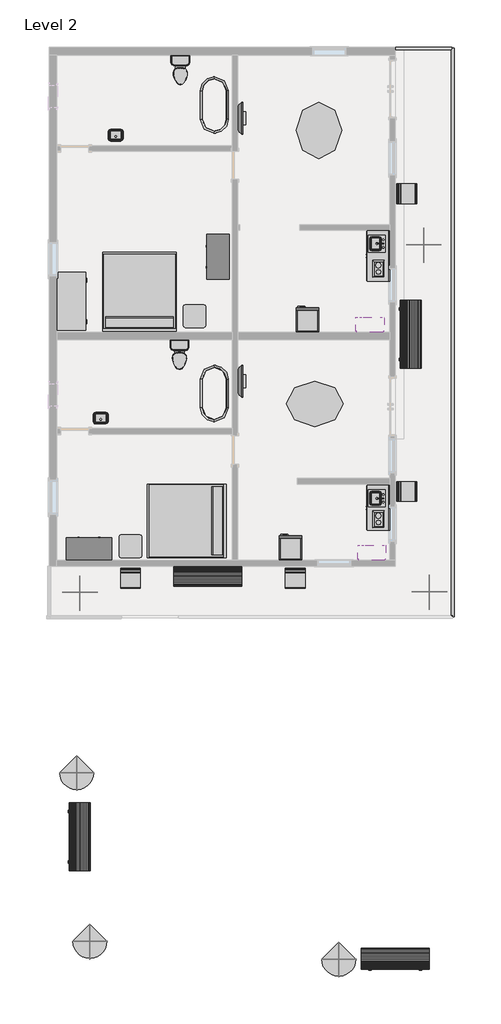
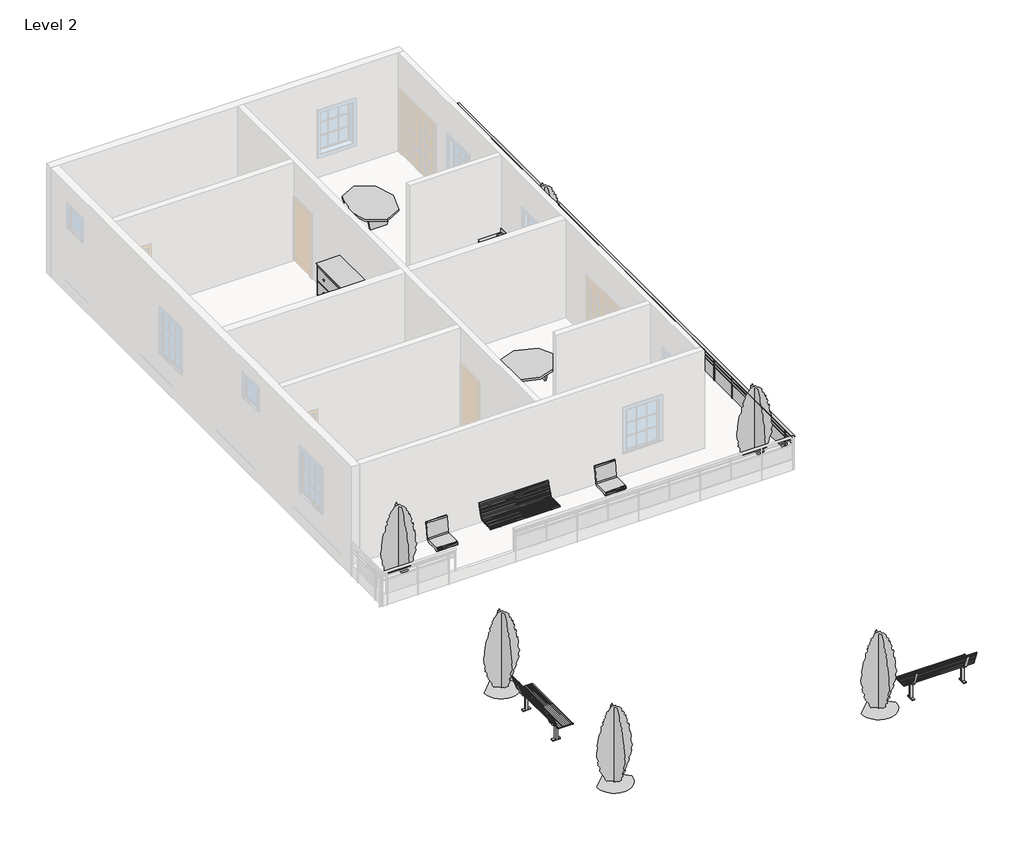
# One storey, part 2 of 2: 17 furniture elements, 10 geographic elements, 8 flow terminals, 8 proxies, 2 railings.
"""IFC4 building model written with IfcOpenShell, lengths in millimetres."""

from ifc_helpers import new_model, si_unit, point, frame, origin, place, context, project, spatial, polyline, ellipse_curve, trimmed, outline, extrude, transform, mapped, element, save
from ifc_brep_helpers import plane_surface, extruded_surface, advanced_brep
from components import proxy_fe84b772, proxy_631763f9, kitchenette_medium_kitchenette_medium_844211aa, m_refrigerator_600_x_660mm_a466bf94, proxy_8a8d5ab2, flow_terminal_871c2e40, toilet_domestic_3d_toilet_domestic_3d_f7549cf7, toilet_domestic_3d_toilet_domestic_3d_183bbd19, flow_terminal_b374fae2, flow_terminal_f2f0329d, furniture_29cd36cd, chair_task_chair_task_b7f3823b, furniture_95afb093, furniture_21562906, furniture_013ab306, furniture_9fa109b2, furniture_56245f3a, furniture_743965d2, furniture_bcf351fa, geographic_element_235d1464, rpc_tree_conifer_chinese_juniper_7_1b9786cd

model = new_model("IFC4")

# Units and contexts
model_context = context("Model", 3, world=origin())
ifc_project = project(units=[si_unit("LENGTHUNIT", "METRE", prefix="MILLI")], contexts=[model_context])

# Site, building, storey
site = spatial("IfcSite", under=ifc_project)
building = spatial("IfcBuilding", under=site)
storey = spatial("IfcBuildingStorey", under=building, Name="Level 2", Elevation=3048.0)

# Proxies
placement = place(None, origin())
proxy_shape = proxy_fe84b772(model_context)
element("IfcBuildingElementProxy", 1, Name="Cook Top-2 Unit : 12\" x 18\"", ObjectType="Cook Top-2 Unit : 12\" x 18\"", at=placement, inside=storey, context=model_context, shape_type="MappedRepresentation", body=[
    mapped(proxy_shape, transform((-224.0170266, 6907.0675398, 3048.0), x_axis=(1.0000000000000004, 0.0, 0.0), y_axis=(0.0, 1.0000000000000004, 0.0), z_axis=(0.0, 0.0, 1.0))),
])
element("IfcBuildingElementProxy", 2, Name="Cook Top-2 Unit : 12\" x 18\"", ObjectType="Cook Top-2 Unit : 12\" x 18\"", at=placement, inside=storey, context=model_context, shape_type="MappedRepresentation", body=[
    mapped(proxy_shape, transform((-224.0170266, 157.3298349, 3048.0), x_axis=(1.0, 0.0, 0.0), y_axis=(0.0, 1.0, 0.0), z_axis=(0.0, 0.0, 1.0))),
])
proxy_2_shape = proxy_631763f9(model_context)
element("IfcBuildingElementProxy", 3, Name="Kitchenette - Small : 48\"", ObjectType="Kitchenette - Small : 48\"", at=placement, inside=storey, context=model_context, shape_type="MappedRepresentation", body=[
    mapped(proxy_2_shape, transform((156.9829734, 511.0923354, 3048.0), x_axis=(0.0, -1.0, 0.0), y_axis=(1.0, 0.0, 0.0), z_axis=(0.0, 0.0, 1.0))),
])
kitchenette_medium_kitchenette_medium_shape = kitchenette_medium_kitchenette_medium_844211aa(model_context)
element("IfcBuildingElementProxy", 4, Name="Kitchenette - Small : 54\"", ObjectType="Kitchenette - Small : 54\"", at=placement, inside=storey, context=model_context, shape_type="MappedRepresentation", body=[
    mapped(kitchenette_medium_kitchenette_medium_shape, transform((156.9829734, 7298.9300403, 3048.0), x_axis=(0.0, -1.0000000000000004, 0.0), y_axis=(1.0000000000000004, 0.0, 0.0), z_axis=(0.0, 0.0, 1.0))),
])
m_refrigerator_600_x_660mm_shape = m_refrigerator_600_x_660mm_a466bf94(model_context)
element("IfcBuildingElementProxy", 5, Name="M_Refrigerator : 600 x 660mm", ObjectType="M_Refrigerator : 600 x 660mm", at=placement, inside=storey, context=model_context, shape_type="MappedRepresentation", body=[
    mapped(m_refrigerator_600_x_660mm_shape, transform((-2111.4181692, 5519.0074256, 3048.0), x_axis=(-1.0000000000000002, 0.0, 0.0), y_axis=(0.0, -1.0000000000000002, 0.0), z_axis=(0.0, 0.0, 1.0))),
])
element("IfcBuildingElementProxy", 6, Name="M_Refrigerator : 600 x 660mm", ObjectType="M_Refrigerator : 600 x 660mm", at=placement, inside=storey, context=model_context, shape_type="MappedRepresentation", body=[
    mapped(m_refrigerator_600_x_660mm_shape, transform((-2568.6181692, -627.7925744, 3048.0), x_axis=(-1.0, 0.0, 0.0), y_axis=(0.0, -1.0, 0.0), z_axis=(0.0, 0.0, 1.0))),
])
proxy_3_shape = proxy_8a8d5ab2(model_context)
element("IfcBuildingElementProxy", 7, Name="Microwave : 30\" x 16\" x 18\"", ObjectType="Microwave : 30\" x 16\" x 18\"", at=placement, inside=storey, context=model_context, shape_type="MappedRepresentation", body=[
    mapped(proxy_3_shape, transform((123.8758508, 5072.9118296, 3352.8), x_axis=(-1.0000000000000004, 0.0, 0.0), y_axis=(0.0, -1.0000000000000004, 0.0), z_axis=(0.0, 0.0, 1.0))),
])
element("IfcBuildingElementProxy", 8, Name="Microwave : 30\" x 16\" x 18\"", ObjectType="Microwave : 30\" x 16\" x 18\"", at=placement, inside=storey, context=model_context, shape_type="MappedRepresentation", body=[
    mapped(proxy_3_shape, transform((174.6758508, -1073.8881704, 3352.8), x_axis=(-1.0000000000000004, 0.0, 0.0), y_axis=(0.0, -1.0000000000000004, 0.0), z_axis=(0.0, 0.0, 1.0))),
])

# Flow terminals
flow_terminal_shape = flow_terminal_871c2e40(model_context)
element("IfcFlowTerminal", 9, ObjectType="Sink Kitchen-Island : 18\" x 18\"", at=placement, inside=storey, context=model_context, shape_type="MappedRepresentation", body=[
    mapped(flow_terminal_shape, transform((-7206.027786, 10495.6377365, 3352.8), x_axis=(-1.0000000000000004, 0.0, 0.0), y_axis=(0.0, -1.0000000000000004, 0.0), z_axis=(0.0, 0.0, 1.0))),
])
element("IfcFlowTerminal", 10, ObjectType="Sink Kitchen-Island : 18\" x 18\"", at=placement, inside=storey, context=model_context, shape_type="MappedRepresentation", body=[
    mapped(flow_terminal_shape, transform((-7612.427786, 2875.6377365, 3352.8), x_axis=(-1.0, 0.0, 0.0), y_axis=(0.0, -1.0, 0.0), z_axis=(0.0, 0.0, 1.0))),
])
element("IfcFlowTerminal", 11, ObjectType="Sink Kitchen-Island : 18\" x 18\"", at=placement, inside=storey, context=model_context, shape_type="MappedRepresentation", body=[
    mapped(flow_terminal_shape, transform((-188.2624277, 7626.081576, 3048.0), x_axis=(0.0, -1.0000000000000004, 0.0), y_axis=(1.0000000000000004, 0.0, 0.0), z_axis=(0.0, 0.0, 1.0))),
])
element("IfcFlowTerminal", 12, ObjectType="Sink Kitchen-Island : 18\" x 18\"", at=placement, inside=storey, context=model_context, shape_type="MappedRepresentation", body=[
    mapped(flow_terminal_shape, transform((-188.2624277, 762.0438711, 3048.0), x_axis=(0.0, -1.0, 0.0), y_axis=(1.0, 0.0, 0.0), z_axis=(0.0, 0.0, 1.0))),
])
toilet_domestic_3d_toilet_domestic_3d_shape = toilet_domestic_3d_toilet_domestic_3d_f7549cf7(model_context)
toilet_domestic_3d_toilet_domestic_3d_2_shape = toilet_domestic_3d_toilet_domestic_3d_183bbd19(model_context)
element("IfcFlowTerminal", 13, ObjectType="Toilet-Domestic-3D : Toilet-Domestic-3D", at=placement, inside=storey, context=model_context, shape_type="MappedRepresentation", body=[
    mapped(toilet_domestic_3d_toilet_domestic_3d_shape, transform((-5481.8170266, 12195.6963081, 3048.0), x_axis=(1.0, 0.0, 0.0), y_axis=(0.0, 1.0, 0.0), z_axis=(0.0, 0.0, 1.0))),
    mapped(toilet_domestic_3d_toilet_domestic_3d_2_shape, transform((-5481.8170266, 12195.6963081, 3048.0), x_axis=(1.0, 0.0, 0.0), y_axis=(0.0, 1.0, 0.0), z_axis=(0.0, 0.0, 1.0))),
])
element("IfcFlowTerminal", 14, ObjectType="Toilet-Domestic-3D : Toilet-Domestic-3D", at=placement, inside=storey, context=model_context, shape_type="MappedRepresentation", body=[
    mapped(toilet_domestic_3d_toilet_domestic_3d_shape, transform((-5507.2170266, 4524.8963081, 3048.0), x_axis=(1.0, 0.0, 0.0), y_axis=(0.0, 1.0, 0.0), z_axis=(0.0, 0.0, 1.0))),
    mapped(toilet_domestic_3d_toilet_domestic_3d_2_shape, transform((-5507.2170266, 4524.8963081, 3048.0), x_axis=(1.0, 0.0, 0.0), y_axis=(0.0, 1.0, 0.0), z_axis=(0.0, 0.0, 1.0))),
])
flow_terminal_2_shape = flow_terminal_b374fae2(model_context)
element("IfcFlowTerminal", 15, ObjectType="Tub-Free Standing-3D : 30\" x 60\"", at=placement, inside=storey, context=model_context, shape_type="MappedRepresentation", body=[
    mapped(flow_terminal_2_shape, transform((-4567.4170266, 3571.7923354, 3048.0), x_axis=(1.0, 0.0, 0.0), y_axis=(0.0, 1.0, 0.0), z_axis=(0.0, 0.0, 1.0))),
])
flow_terminal_3_shape = flow_terminal_f2f0329d(model_context)
element("IfcFlowTerminal", 16, ObjectType="Tub-Free Standing-3D : 30\" x 60\"", at=placement, inside=storey, context=model_context, shape_type="MappedRepresentation", body=[
    mapped(flow_terminal_3_shape, transform((-4567.4170266, 11344.1923354, 3048.0), x_axis=(-1.0, 0.0, 0.0), y_axis=(0.0, -1.0, 0.0), z_axis=(0.0, 0.0, 1.0))),
])

# Furniture
furniture_shape = furniture_29cd36cd(model_context)
element("IfcFurniture", 17, ObjectType="Bed-Shaker : King 78\" x 83\"", at=placement, inside=storey, context=model_context, shape_type="MappedRepresentation", body=[
    mapped(furniture_shape, transform((-6603.1645676, 5267.7628272, 3048.0), x_axis=(-1.0000000000000002, 0.0, 0.0), y_axis=(0.0, -1.0000000000000002, 0.0), z_axis=(0.0, 0.0, 1.0))),
])
element("IfcFurniture", 18, ObjectType="Bed-Shaker : King 78\" x 83\"", at=placement, inside=storey, context=model_context, shape_type="MappedRepresentation", body=[
    mapped(furniture_shape, transform((-4262.6170266, 123.7423354, 3048.0), x_axis=(0.0, -1.0, 0.0), y_axis=(1.0, 0.0, 0.0), z_axis=(0.0, 0.0, 1.0))),
])
chair_task_chair_task_shape = chair_task_chair_task_b7f3823b(model_context)
element("IfcFurniture", 19, ObjectType="Chair-Task : Chair-Task", at=placement, inside=storey, context=model_context, shape_type="MappedRepresentation", body=[
    mapped(chair_task_chair_task_shape, transform((-2242.0262069, -1387.6617629, 3048.0), x_axis=(-1.0000000000000004, 0.0, 0.0), y_axis=(0.0, -1.0000000000000004, 0.0), z_axis=(0.0, 0.0, 1.0))),
])
element("IfcFurniture", 20, ObjectType="Chair-Task : Chair-Task", at=placement, inside=storey, context=model_context, shape_type="MappedRepresentation", body=[
    mapped(chair_task_chair_task_shape, transform((-6687.0262069, -1387.6617629, 3048.0), x_axis=(-1.0000000000000004, 0.0, 0.0), y_axis=(0.0, -1.0000000000000004, 0.0), z_axis=(0.0, 0.0, 1.0))),
])
element("IfcFurniture", 21, ObjectType="Chair-Task : Chair-Task", at=placement, inside=storey, context=model_context, shape_type="MappedRepresentation", body=[
    mapped(chair_task_chair_task_shape, transform((595.2370718, 1071.1831551, 3048.0), x_axis=(0.0, -1.0000000000000007, 0.0), y_axis=(1.0000000000000007, 0.0, 0.0), z_axis=(0.0, 0.0, 1.0))),
])
element("IfcFurniture", 22, ObjectType="Chair-Task : Chair-Task", at=placement, inside=storey, context=model_context, shape_type="MappedRepresentation", body=[
    mapped(chair_task_chair_task_shape, transform((595.2370718, 9097.5831551, 3048.0), x_axis=(0.0, -1.0000000000000007, 0.0), y_axis=(1.0000000000000007, 0.0, 0.0), z_axis=(0.0, 0.0, 1.0))),
])
furniture_2_shape = furniture_95afb093(model_context)
element("IfcFurniture", 23, ObjectType="Counter Top w Sink Hole : 24\" Depth", at=placement, inside=storey, context=model_context, shape_type="MappedRepresentation", body=[
    mapped(furniture_2_shape, transform((156.9829734, 6765.5300403, 3048.0), x_axis=(0.0, -1.0000000000000004, 0.0), y_axis=(1.0000000000000004, 0.0, 0.0), z_axis=(0.0, 0.0, 1.0))),
])
furniture_3_shape = furniture_21562906(model_context)
element("IfcFurniture", 24, ObjectType="Counter Top w Sink Hole : 24\" Depth", at=placement, inside=storey, context=model_context, shape_type="MappedRepresentation", body=[
    mapped(furniture_3_shape, transform((156.9829734, -98.5076646, 3048.0), x_axis=(0.0, -1.0, 0.0), y_axis=(1.0, 0.0, 0.0), z_axis=(0.0, 0.0, 1.0))),
])
furniture_4_shape = furniture_013ab306(model_context)
element("IfcFurniture", 25, ObjectType="Desk : 60\" x 30\" Student", at=placement, inside=storey, context=model_context, shape_type="MappedRepresentation", body=[
    mapped(furniture_4_shape, transform((-8047.2170266, 5298.9923354, 3048.0), x_axis=(0.0, 1.0000000000000002, 0.0), y_axis=(-1.0000000000000002, 0.0, 0.0), z_axis=(0.0, 0.0, 1.0))),
])
furniture_5_shape = furniture_9fa109b2(model_context)
element("IfcFurniture", 26, ObjectType="Dresser : 48\" x 72\" x 24\"", at=placement, inside=storey, context=model_context, shape_type="MappedRepresentation", body=[
    mapped(furniture_5_shape, transform((-4102.6540725, 6985.5990756, 3048.0), x_axis=(0.0, -1.0, 0.0), y_axis=(1.0, 0.0, 0.0), z_axis=(0.0, 0.0, 1.0))),
])
element("IfcFurniture", 27, ObjectType="Dresser : 48\" x 72\" x 24\"", at=placement, inside=storey, context=model_context, shape_type="MappedRepresentation", body=[
    mapped(furniture_5_shape, transform((-8214.8102864, -982.3706187, 3048.0), x_axis=(-1.0000000000000004, 0.0, 0.0), y_axis=(0.0, -1.0000000000000004, 0.0), z_axis=(0.0, 0.0, 1.0))),
])
furniture_6_shape = furniture_56245f3a(model_context)
element("IfcFurniture", 28, ObjectType="TV - Flat Screen : 32\"", at=placement, inside=storey, context=model_context, shape_type="MappedRepresentation", body=[
    mapped(furniture_6_shape, transform((-3873.8784029, 3905.9368496, 3962.4), x_axis=(0.0, 1.0000000000000009, 0.0), y_axis=(-1.0000000000000009, 0.0, 0.0), z_axis=(0.0, 0.0, 1.0))),
])
element("IfcFurniture", 29, ObjectType="TV - Flat Screen : 32\"", at=placement, inside=storey, context=model_context, shape_type="MappedRepresentation", body=[
    mapped(furniture_6_shape, transform((-3873.8784029, 10992.5368496, 3962.4), x_axis=(0.0, 1.0000000000000002, 0.0), y_axis=(-1.0000000000000002, 0.0, 0.0), z_axis=(0.0, 0.0, 1.0))),
])
furniture_7_shape = furniture_743965d2(model_context)
element("IfcFurniture", 30, ObjectType="Table-Ellipse : 60\" x 48\"", at=placement, inside=storey, context=model_context, shape_type="MappedRepresentation", body=[
    mapped(furniture_7_shape, transform((-1862.3170266, 3292.3923354, 3048.0), x_axis=(1.0, 0.0, 0.0), y_axis=(0.0, 1.0, 0.0), z_axis=(0.0, 0.0, 1.0))),
])
element("IfcFurniture", 31, ObjectType="Table-Ellipse : 60\" x 48\"", at=placement, inside=storey, context=model_context, shape_type="MappedRepresentation", body=[
    mapped(furniture_7_shape, transform((-1748.0170266, 10658.3923354, 3048.0), x_axis=(0.0, 1.0, 0.0), y_axis=(-1.0, 0.0, 0.0), z_axis=(0.0, 0.0, 1.0))),
])
furniture_8_shape = furniture_bcf351fa(model_context)
element("IfcFurniture", 32, ObjectType="Table-End : 24\" x 24\"", at=placement, inside=storey, context=model_context, shape_type="MappedRepresentation", body=[
    mapped(furniture_8_shape, transform((-5409.3506569, 5502.1923354, 3048.0), x_axis=(1.0, 0.0, 0.0), y_axis=(0.0, 1.0, 0.0), z_axis=(0.0, 0.0, 1.0))),
])
element("IfcFurniture", 33, ObjectType="Table-End : 24\" x 24\"", at=placement, inside=storey, context=model_context, shape_type="MappedRepresentation", body=[
    mapped(furniture_8_shape, transform((-7136.5506569, -695.4076646, 3048.0), x_axis=(1.0, 0.0, 0.0), y_axis=(0.0, 1.0, 0.0), z_axis=(0.0, 0.0, 1.0))),
])

# Geographic elements
geographic_element_shape = geographic_element_235d1464(model_context)
element("IfcGeographicElement", 34, ObjectType="Park Bench : 72\"", at=placement, inside=storey, context=model_context, shape_type="MappedRepresentation", body=[
    mapped(geographic_element_shape, transform((-4745.2170266, -1305.0076646, 3048.0), x_axis=(1.0, 0.0, 0.0), y_axis=(0.0, 1.0, 0.0), z_axis=(0.0, 0.0, 1.0))),
])
element("IfcGeographicElement", 35, ObjectType="Park Bench : 72\"", at=placement, inside=storey, context=model_context, shape_type="MappedRepresentation", body=[
    mapped(geographic_element_shape, transform((690.3829734, 5171.9923354, 3048.0), x_axis=(0.0, 1.0000000000000002, 0.0), y_axis=(-1.0000000000000002, 0.0, 0.0), z_axis=(0.0, 0.0, 1.0))),
])
element("IfcGeographicElement", 36, ObjectType="Park Bench : 72\"", at=placement, inside=storey, context=model_context, shape_type="MappedRepresentation", body=[
    mapped(geographic_element_shape, transform((-8225.0170266, -8366.2076646, 3048.0), x_axis=(0.0, 1.0, 0.0), y_axis=(-1.0, 0.0, 0.0), z_axis=(0.0, 0.0, 1.0))),
])
element("IfcGeographicElement", 37, ObjectType="Park Bench : 72\"", at=placement, inside=storey, context=model_context, shape_type="MappedRepresentation", body=[
    mapped(geographic_element_shape, transform((309.3829734, -11693.6076646, 3048.0), x_axis=(-1.0, 0.0, 0.0), y_axis=(0.0, -1.0, 0.0), z_axis=(0.0, 0.0, 1.0))),
])
rpc_tree_conifer_chinese_juniper_7_shape = rpc_tree_conifer_chinese_juniper_7_1b9786cd(model_context)
element("IfcGeographicElement", 38, ObjectType="RPC Tree - Conifer : Chinese Juniper - 7'", at=placement, inside=storey, context=model_context, shape_type="MappedRepresentation", body=[
    mapped(rpc_tree_conifer_chinese_juniper_7_shape, transform((-8193.4636976, -1787.6076646, 3048.0), x_axis=(1.0, 0.0, 0.0), y_axis=(0.0, 1.0, 0.0), z_axis=(0.0, 0.0, 1.0))),
])
element("IfcGeographicElement", 39, ObjectType="RPC Tree - Conifer : Chinese Juniper - 7'", at=placement, inside=storey, context=model_context, shape_type="MappedRepresentation", body=[
    mapped(rpc_tree_conifer_chinese_juniper_7_shape, transform((1223.5863024, -1762.2076646, 3048.0), x_axis=(1.0, 0.0, 0.0), y_axis=(0.0, 1.0, 0.0), z_axis=(0.0, 0.0, 1.0))),
])
element("IfcGeographicElement", 40, ObjectType="RPC Tree - Conifer : Chinese Juniper - 7'", at=placement, inside=storey, context=model_context, shape_type="MappedRepresentation", body=[
    mapped(rpc_tree_conifer_chinese_juniper_7_shape, transform((1071.1863024, 7584.9923354, 3048.0), x_axis=(1.0, 0.0, 0.0), y_axis=(0.0, 1.0, 0.0), z_axis=(0.0, 0.0, 1.0))),
])
element("IfcGeographicElement", 41, ObjectType="RPC Tree - Conifer : Chinese Juniper - 7'", at=placement, inside=storey, context=model_context, shape_type="MappedRepresentation", body=[
    mapped(rpc_tree_conifer_chinese_juniper_7_shape, transform((-7920.4136976, -11185.6076646, 3048.0), x_axis=(1.0, 0.0, 0.0), y_axis=(0.0, 1.0, 0.0), z_axis=(0.0, 0.0, 1.0))),
])
element("IfcGeographicElement", 42, ObjectType="RPC Tree - Conifer : Chinese Juniper - 7'", at=placement, inside=storey, context=model_context, shape_type="MappedRepresentation", body=[
    mapped(rpc_tree_conifer_chinese_juniper_7_shape, transform((-8276.0136976, -6639.0076646, 3048.0), x_axis=(1.0, 0.0, 0.0), y_axis=(0.0, 1.0, 0.0), z_axis=(0.0, 0.0, 1.0))),
])
element("IfcGeographicElement", 43, ObjectType="RPC Tree - Conifer : Chinese Juniper - 7'", at=placement, inside=storey, context=model_context, shape_type="MappedRepresentation", body=[
    mapped(rpc_tree_conifer_chinese_juniper_7_shape, transform((-1214.8136976, -11668.2076646, 3048.0), x_axis=(1.0, 0.0, 0.0), y_axis=(0.0, 1.0, 0.0), z_axis=(0.0, 0.0, 1.0))),
])

# Railings
element("IfcRailing", 44, ObjectType="Glass Panel - Bottom Fill", at=placement, inside=storey, context=model_context, shape_type="SolidModel", body=[
    advanced_brep(
    [(1820.6829734, -2448.0076646, 3962.4), (1896.8829734, -2448.0076646, 3962.4), (1820.6829734, 12868.1923354, 3962.4), (1896.8829734, 12868.1923354, 3962.4)],
    [
        (0, 1, ellipse_curve(frame((1858.7829734, -2448.0076646, 3962.4), z_axis=(0.0, -1.0, 0.0), x_axis=(1.0, 0.0, 0.0)), 38.1, 28.575)),
        (1, 0, ellipse_curve(frame((1858.7829734, -2448.0076646, 3962.4), z_axis=(0.0, -1.0, 0.0), x_axis=(1.0, 0.0, 0.0)), 38.1, 28.575)),
        (2, 3, ellipse_curve(frame((1858.7829734, 12868.1923354, 3962.4), z_axis=(0.0, 1.0, 0.0), x_axis=(1.0, 0.0, 0.0)), 38.1, 28.575)),
        (3, 2, ellipse_curve(frame((1858.7829734, 12868.1923354, 3962.4), z_axis=(0.0, 1.0, 0.0), x_axis=(1.0, 0.0, 0.0)), 38.1, 28.575)),
        (0, 2),
        (3, 1),
    ],
    [
        plane_surface(frame((1858.7829734, -2448.0076646, 3962.4), z_axis=(0.0, -1.0, 0.0), x_axis=(0.0, 0.0, 1.0))),
        plane_surface(frame((1858.7829734, 12868.1923354, 3962.4), z_axis=(0.0, 1.0, 0.0), x_axis=(0.0, 0.0, 1.0))),
        extruded_surface(trimmed(ellipse_curve(frame((1858.7829734, 12868.1923354, 3962.4), z_axis=(0.0, -1.0, 0.0), x_axis=(1.0, 0.0, 0.0)), 38.1, 28.575), [point((1820.6829734, 12868.1923354, 3962.4))], [point((1896.8829734, 12868.1923354, 3962.4))], True, "CARTESIAN"), (0.0, -15316.199999999999, 0.0), 15316.199999999999),
        extruded_surface(trimmed(ellipse_curve(frame((1858.7829734, 12868.1923354, 3962.4), z_axis=(0.0, -1.0, 0.0), x_axis=(1.0, 0.0, 0.0)), 38.1, 28.575), [point((1896.8829734, 12868.1923354, 3962.4))], [point((1820.6829734, 12868.1923354, 3962.4))], True, "CARTESIAN"), (0.0, -15316.199999999999, 0.0), 15316.199999999999),
    ],
    [
        (0, [[1, 2]]),
        (1, [[3, 4]]),
        (2, [[-1, 5, -4, 6]]),
        (3, [[-2, -6, -3, -5]]),
    ],
),
    extrude(outline(polyline([(1871.4829734, -2448.0076646), (1846.0829734, -2448.0076646), (1846.0829734, 12868.1923354), (1871.4829734, 12868.1923354), (1871.4829734, -2448.0076646)])), frame((0.0, 0.0, 3848.1), z_axis=(0.0, 0.0, 1.0), x_axis=(1.0, 0.0, 0.0)), (0.0, 0.0, 1.0), 25.4),
    extrude(outline(polyline([(1871.4829734, -2448.0076646), (1846.0829734, -2448.0076646), (1846.0829734, 12868.1923354), (1871.4829734, 12868.1923354), (1871.4829734, -2448.0076646)])), frame((0.0, 0.0, 3746.5), z_axis=(0.0, 0.0, 1.0), x_axis=(1.0, 0.0, 0.0)), (0.0, 0.0, 1.0), 25.4),
    extrude(outline(polyline([(1884.1829734, 12518.9423354), (1833.3829734, 12518.9423354), (1833.3829734, 12531.6423354), (1884.1829734, 12531.6423354), (1884.1829734, 12518.9423354)])), frame((0.0, 0.0, 3048.0), z_axis=(0.0, 0.0, 1.0), x_axis=(1.0, 0.0, 0.0)), (0.0, 0.0, 1.0), 885.6788223),
    extrude(outline(polyline([(1852.2478164, 11712.4923354), (1852.2478164, 12525.2923354), (1858.5978164, 12525.2923354), (1858.5978164, 11712.4923354), (1852.2478164, 11712.4923354)])), frame((0.0, 0.0, 3149.6), z_axis=(0.0, 0.0, 1.0), x_axis=(1.0, 0.0, 0.0)), (0.0, 0.0, 1.0), 596.9),
    extrude(outline(polyline([(1884.1829734, 11706.1423354), (1833.3829734, 11706.1423354), (1833.3829734, 11718.8423354), (1884.1829734, 11718.8423354), (1884.1829734, 11706.1423354)])), frame((0.0, 0.0, 3048.0), z_axis=(0.0, 0.0, 1.0), x_axis=(1.0, 0.0, 0.0)), (0.0, 0.0, 1.0), 885.6788223),
    extrude(outline(polyline([(1852.2478164, 10899.6923354), (1852.2478164, 11712.4923354), (1858.5978164, 11712.4923354), (1858.5978164, 10899.6923354), (1852.2478164, 10899.6923354)])), frame((0.0, 0.0, 3149.6), z_axis=(0.0, 0.0, 1.0), x_axis=(1.0, 0.0, 0.0)), (0.0, 0.0, 1.0), 596.9),
    extrude(outline(polyline([(1884.1829734, 10893.3423354), (1833.3829734, 10893.3423354), (1833.3829734, 10906.0423354), (1884.1829734, 10906.0423354), (1884.1829734, 10893.3423354)])), frame((0.0, 0.0, 3048.0), z_axis=(0.0, 0.0, 1.0), x_axis=(1.0, 0.0, 0.0)), (0.0, 0.0, 1.0), 885.6788223),
    extrude(outline(polyline([(1852.2478164, 10086.8923354), (1852.2478164, 10899.6923354), (1858.5978164, 10899.6923354), (1858.5978164, 10086.8923354), (1852.2478164, 10086.8923354)])), frame((0.0, 0.0, 3149.6), z_axis=(0.0, 0.0, 1.0), x_axis=(1.0, 0.0, 0.0)), (0.0, 0.0, 1.0), 596.9),
    extrude(outline(polyline([(1884.1829734, 10080.5423354), (1833.3829734, 10080.5423354), (1833.3829734, 10093.2423354), (1884.1829734, 10093.2423354), (1884.1829734, 10080.5423354)])), frame((0.0, 0.0, 3048.0), z_axis=(0.0, 0.0, 1.0), x_axis=(1.0, 0.0, 0.0)), (0.0, 0.0, 1.0), 885.6788223),
    extrude(outline(polyline([(1852.2478164, 9274.0923354), (1852.2478164, 10086.8923354), (1858.5978164, 10086.8923354), (1858.5978164, 9274.0923354), (1852.2478164, 9274.0923354)])), frame((0.0, 0.0, 3149.6), z_axis=(0.0, 0.0, 1.0), x_axis=(1.0, 0.0, 0.0)), (0.0, 0.0, 1.0), 596.9),
    extrude(outline(polyline([(1884.1829734, 9267.7423354), (1833.3829734, 9267.7423354), (1833.3829734, 9280.4423354), (1884.1829734, 9280.4423354), (1884.1829734, 9267.7423354)])), frame((0.0, 0.0, 3048.0), z_axis=(0.0, 0.0, 1.0), x_axis=(1.0, 0.0, 0.0)), (0.0, 0.0, 1.0), 885.6788223),
    extrude(outline(polyline([(1852.2478164, 8461.2923354), (1852.2478164, 9274.0923354), (1858.5978164, 9274.0923354), (1858.5978164, 8461.2923354), (1852.2478164, 8461.2923354)])), frame((0.0, 0.0, 3149.6), z_axis=(0.0, 0.0, 1.0), x_axis=(1.0, 0.0, 0.0)), (0.0, 0.0, 1.0), 596.9),
    extrude(outline(polyline([(1884.1829734, 8454.9423354), (1833.3829734, 8454.9423354), (1833.3829734, 8467.6423354), (1884.1829734, 8467.6423354), (1884.1829734, 8454.9423354)])), frame((0.0, 0.0, 3048.0), z_axis=(0.0, 0.0, 1.0), x_axis=(1.0, 0.0, 0.0)), (0.0, 0.0, 1.0), 885.6788223),
    extrude(outline(polyline([(1852.2478164, 7648.4923354), (1852.2478164, 8461.2923354), (1858.5978164, 8461.2923354), (1858.5978164, 7648.4923354), (1852.2478164, 7648.4923354)])), frame((0.0, 0.0, 3149.6), z_axis=(0.0, 0.0, 1.0), x_axis=(1.0, 0.0, 0.0)), (0.0, 0.0, 1.0), 596.9),
    extrude(outline(polyline([(1884.1829734, 7642.1423354), (1833.3829734, 7642.1423354), (1833.3829734, 7654.8423354), (1884.1829734, 7654.8423354), (1884.1829734, 7642.1423354)])), frame((0.0, 0.0, 3048.0), z_axis=(0.0, 0.0, 1.0), x_axis=(1.0, 0.0, 0.0)), (0.0, 0.0, 1.0), 885.6788223),
    extrude(outline(polyline([(1852.2478164, 6835.6923354), (1852.2478164, 7648.4923354), (1858.5978164, 7648.4923354), (1858.5978164, 6835.6923354), (1852.2478164, 6835.6923354)])), frame((0.0, 0.0, 3149.6), z_axis=(0.0, 0.0, 1.0), x_axis=(1.0, 0.0, 0.0)), (0.0, 0.0, 1.0), 596.9),
    extrude(outline(polyline([(1884.1829734, 6829.3423354), (1833.3829734, 6829.3423354), (1833.3829734, 6842.0423354), (1884.1829734, 6842.0423354), (1884.1829734, 6829.3423354)])), frame((0.0, 0.0, 3048.0), z_axis=(0.0, 0.0, 1.0), x_axis=(1.0, 0.0, 0.0)), (0.0, 0.0, 1.0), 885.6788223),
    extrude(outline(polyline([(1852.2478164, 6022.8923354), (1852.2478164, 6835.6923354), (1858.5978164, 6835.6923354), (1858.5978164, 6022.8923354), (1852.2478164, 6022.8923354)])), frame((0.0, 0.0, 3149.6), z_axis=(0.0, 0.0, 1.0), x_axis=(1.0, 0.0, 0.0)), (0.0, 0.0, 1.0), 596.9),
    extrude(outline(polyline([(1884.1829734, 6016.5423354), (1833.3829734, 6016.5423354), (1833.3829734, 6029.2423354), (1884.1829734, 6029.2423354), (1884.1829734, 6016.5423354)])), frame((0.0, 0.0, 3048.0), z_axis=(0.0, 0.0, 1.0), x_axis=(1.0, 0.0, 0.0)), (0.0, 0.0, 1.0), 885.6788223),
    extrude(outline(polyline([(1852.2478164, 5210.0923354), (1852.2478164, 6022.8923354), (1858.5978164, 6022.8923354), (1858.5978164, 5210.0923354), (1852.2478164, 5210.0923354)])), frame((0.0, 0.0, 3149.6), z_axis=(0.0, 0.0, 1.0), x_axis=(1.0, 0.0, 0.0)), (0.0, 0.0, 1.0), 596.9),
    extrude(outline(polyline([(1884.1829734, 5203.7423354), (1833.3829734, 5203.7423354), (1833.3829734, 5216.4423354), (1884.1829734, 5216.4423354), (1884.1829734, 5203.7423354)])), frame((0.0, 0.0, 3048.0), z_axis=(0.0, 0.0, 1.0), x_axis=(1.0, 0.0, 0.0)), (0.0, 0.0, 1.0), 885.6788223),
    extrude(outline(polyline([(1852.2478164, 4397.2923354), (1852.2478164, 5210.0923354), (1858.5978164, 5210.0923354), (1858.5978164, 4397.2923354), (1852.2478164, 4397.2923354)])), frame((0.0, 0.0, 3149.6), z_axis=(0.0, 0.0, 1.0), x_axis=(1.0, 0.0, 0.0)), (0.0, 0.0, 1.0), 596.9),
    extrude(outline(polyline([(1884.1829734, 4390.9423354), (1833.3829734, 4390.9423354), (1833.3829734, 4403.6423354), (1884.1829734, 4403.6423354), (1884.1829734, 4390.9423354)])), frame((0.0, 0.0, 3048.0), z_axis=(0.0, 0.0, 1.0), x_axis=(1.0, 0.0, 0.0)), (0.0, 0.0, 1.0), 885.6788223),
    extrude(outline(polyline([(1852.2478164, 3584.4923354), (1852.2478164, 4397.2923354), (1858.5978164, 4397.2923354), (1858.5978164, 3584.4923354), (1852.2478164, 3584.4923354)])), frame((0.0, 0.0, 3149.6), z_axis=(0.0, 0.0, 1.0), x_axis=(1.0, 0.0, 0.0)), (0.0, 0.0, 1.0), 596.9),
    extrude(outline(polyline([(1884.1829734, 3578.1423354), (1833.3829734, 3578.1423354), (1833.3829734, 3590.8423354), (1884.1829734, 3590.8423354), (1884.1829734, 3578.1423354)])), frame((0.0, 0.0, 3048.0), z_axis=(0.0, 0.0, 1.0), x_axis=(1.0, 0.0, 0.0)), (0.0, 0.0, 1.0), 885.6788223),
    extrude(outline(polyline([(1852.2478164, 2771.6923354), (1852.2478164, 3584.4923354), (1858.5978164, 3584.4923354), (1858.5978164, 2771.6923354), (1852.2478164, 2771.6923354)])), frame((0.0, 0.0, 3149.6), z_axis=(0.0, 0.0, 1.0), x_axis=(1.0, 0.0, 0.0)), (0.0, 0.0, 1.0), 596.9),
    extrude(outline(polyline([(1884.1829734, 2765.3423354), (1833.3829734, 2765.3423354), (1833.3829734, 2778.0423354), (1884.1829734, 2778.0423354), (1884.1829734, 2765.3423354)])), frame((0.0, 0.0, 3048.0), z_axis=(0.0, 0.0, 1.0), x_axis=(1.0, 0.0, 0.0)), (0.0, 0.0, 1.0), 885.6788223),
    extrude(outline(polyline([(1852.2478164, 1958.8923354), (1852.2478164, 2771.6923354), (1858.5978164, 2771.6923354), (1858.5978164, 1958.8923354), (1852.2478164, 1958.8923354)])), frame((0.0, 0.0, 3149.6), z_axis=(0.0, 0.0, 1.0), x_axis=(1.0, 0.0, 0.0)), (0.0, 0.0, 1.0), 596.9),
    extrude(outline(polyline([(1884.1829734, 1952.5423354), (1833.3829734, 1952.5423354), (1833.3829734, 1965.2423354), (1884.1829734, 1965.2423354), (1884.1829734, 1952.5423354)])), frame((0.0, 0.0, 3048.0), z_axis=(0.0, 0.0, 1.0), x_axis=(1.0, 0.0, 0.0)), (0.0, 0.0, 1.0), 885.6788223),
    extrude(outline(polyline([(1852.2478164, 1146.0923354), (1852.2478164, 1958.8923354), (1858.5978164, 1958.8923354), (1858.5978164, 1146.0923354), (1852.2478164, 1146.0923354)])), frame((0.0, 0.0, 3149.6), z_axis=(0.0, 0.0, 1.0), x_axis=(1.0, 0.0, 0.0)), (0.0, 0.0, 1.0), 596.9),
    extrude(outline(polyline([(1884.1829734, 1139.7423354), (1833.3829734, 1139.7423354), (1833.3829734, 1152.4423354), (1884.1829734, 1152.4423354), (1884.1829734, 1139.7423354)])), frame((0.0, 0.0, 3048.0), z_axis=(0.0, 0.0, 1.0), x_axis=(1.0, 0.0, 0.0)), (0.0, 0.0, 1.0), 885.6788223),
    extrude(outline(polyline([(1852.2478164, 333.2923354), (1852.2478164, 1146.0923354), (1858.5978164, 1146.0923354), (1858.5978164, 333.2923354), (1852.2478164, 333.2923354)])), frame((0.0, 0.0, 3149.6), z_axis=(0.0, 0.0, 1.0), x_axis=(1.0, 0.0, 0.0)), (0.0, 0.0, 1.0), 596.9),
    extrude(outline(polyline([(1884.1829734, 326.9423354), (1833.3829734, 326.9423354), (1833.3829734, 339.6423354), (1884.1829734, 339.6423354), (1884.1829734, 326.9423354)])), frame((0.0, 0.0, 3048.0), z_axis=(0.0, 0.0, 1.0), x_axis=(1.0, 0.0, 0.0)), (0.0, 0.0, 1.0), 885.6788223),
    extrude(outline(polyline([(1852.2478164, -479.5076646), (1852.2478164, 333.2923354), (1858.5978164, 333.2923354), (1858.5978164, -479.5076646), (1852.2478164, -479.5076646)])), frame((0.0, 0.0, 3149.6), z_axis=(0.0, 0.0, 1.0), x_axis=(1.0, 0.0, 0.0)), (0.0, 0.0, 1.0), 596.9),
    extrude(outline(polyline([(1884.1829734, -485.8576646), (1833.3829734, -485.8576646), (1833.3829734, -473.1576646), (1884.1829734, -473.1576646), (1884.1829734, -485.8576646)])), frame((0.0, 0.0, 3048.0), z_axis=(0.0, 0.0, 1.0), x_axis=(1.0, 0.0, 0.0)), (0.0, 0.0, 1.0), 885.6788223),
    extrude(outline(polyline([(1852.2478164, -1292.3076646), (1852.2478164, -479.5076646), (1858.5978164, -479.5076646), (1858.5978164, -1292.3076646), (1852.2478164, -1292.3076646)])), frame((0.0, 0.0, 3149.6), z_axis=(0.0, 0.0, 1.0), x_axis=(1.0, 0.0, 0.0)), (0.0, 0.0, 1.0), 596.9),
    extrude(outline(polyline([(1884.1829734, -1298.6576646), (1833.3829734, -1298.6576646), (1833.3829734, -1285.9576646), (1884.1829734, -1285.9576646), (1884.1829734, -1298.6576646)])), frame((0.0, 0.0, 3048.0), z_axis=(0.0, 0.0, 1.0), x_axis=(1.0, 0.0, 0.0)), (0.0, 0.0, 1.0), 885.6788223),
    extrude(outline(polyline([(1852.2478164, -2105.1076646), (1852.2478164, -1292.3076646), (1858.5978164, -1292.3076646), (1858.5978164, -2105.1076646), (1852.2478164, -2105.1076646)])), frame((0.0, 0.0, 3149.6), z_axis=(0.0, 0.0, 1.0), x_axis=(1.0, 0.0, 0.0)), (0.0, 0.0, 1.0), 596.9),
    extrude(outline(polyline([(1884.1829734, -2111.4576646), (1833.3829734, -2111.4576646), (1833.3829734, -2098.7576646), (1884.1829734, -2098.7576646), (1884.1829734, -2111.4576646)])), frame((0.0, 0.0, 3048.0), z_axis=(0.0, 0.0, 1.0), x_axis=(1.0, 0.0, 0.0)), (0.0, 0.0, 1.0), 885.6788223),
    extrude(outline(polyline([(1868.3079734, 12855.4923354), (1849.2579734, 12855.4923354), (1849.2579734, 12874.5423354), (1868.3079734, 12874.5423354), (1868.3079734, 12855.4923354)])), frame((0.0, 0.0, 3048.0), z_axis=(0.0, 0.0, 1.0), x_axis=(1.0, 0.0, 0.0)), (0.0, 0.0, 1.0), 885.6788223),
    extrude(outline(polyline([(1868.3079734, -2454.3576646), (1849.2579734, -2454.3576646), (1849.2579734, -2435.3076646), (1868.3079734, -2435.3076646), (1868.3079734, -2454.3576646)])), frame((0.0, 0.0, 3048.0), z_axis=(0.0, 0.0, 1.0), x_axis=(1.0, 0.0, 0.0)), (0.0, 0.0, 1.0), 885.6788223),
])
element("IfcRailing", 45, ObjectType="Glass Panel - Bottom Fill", at=placement, inside=storey, context=model_context, shape_type="SolidModel", body=[
    advanced_brep(
    [(1833.3829734, 12830.0923354, 3962.4), (1833.3829734, 12906.2923354, 3962.4), (283.9829734, 12830.0923354, 3962.4), (283.9829734, 12906.2923354, 3962.4)],
    [
        (0, 1, ellipse_curve(frame((1833.3829734, 12868.1923354, 3962.4), z_axis=(1.0, 0.0, 0.0), x_axis=(0.0, 1.0, 0.0)), 38.1, 28.575)),
        (1, 0, ellipse_curve(frame((1833.3829734, 12868.1923354, 3962.4), z_axis=(1.0, 0.0, 0.0), x_axis=(0.0, 1.0, 0.0)), 38.1, 28.575)),
        (2, 3, ellipse_curve(frame((283.9829734, 12868.1923354, 3962.4), z_axis=(-1.0, 0.0, 0.0), x_axis=(0.0, 1.0, 0.0)), 38.1, 28.575)),
        (3, 2, ellipse_curve(frame((283.9829734, 12868.1923354, 3962.4), z_axis=(-1.0, 0.0, 0.0), x_axis=(0.0, 1.0, 0.0)), 38.1, 28.575)),
        (0, 2),
        (3, 1),
    ],
    [
        plane_surface(frame((1833.3829734, 12868.1923354, 3962.4), z_axis=(1.0, 0.0, 0.0), x_axis=(0.0, -1.0, 0.0))),
        plane_surface(frame((283.9829734, 12868.1923354, 3962.4), z_axis=(-1.0, 0.0, 0.0), x_axis=(0.0, -1.0, 0.0))),
        extruded_surface(trimmed(ellipse_curve(frame((283.9829734, 12868.1923354, 3962.4), z_axis=(1.0, 0.0, 0.0), x_axis=(0.0, 1.0, 0.0)), 38.1, 28.575), [point((283.9829734, 12830.0923354, 3962.4))], [point((283.9829734, 12906.2923354, 3962.4))], True, "CARTESIAN"), (1549.4, 0.0, 0.0), 1549.4),
        extruded_surface(trimmed(ellipse_curve(frame((283.9829734, 12868.1923354, 3962.4), z_axis=(1.0, 0.0, 0.0), x_axis=(0.0, 1.0, 0.0)), 38.1, 28.575), [point((283.9829734, 12906.2923354, 3962.4))], [point((283.9829734, 12830.0923354, 3962.4))], True, "CARTESIAN"), (1549.4, 0.0, 0.0), 1549.4),
    ],
    [
        (0, [[1, 2]]),
        (1, [[3, 4]]),
        (2, [[-1, 5, -4, 6]]),
        (3, [[-2, -6, -3, -5]]),
    ],
),
    extrude(outline(polyline([(1833.3829734, 12880.8923354), (1833.3829734, 12855.4923354), (283.9829734, 12855.4923354), (283.9829734, 12880.8923354), (1833.3829734, 12880.8923354)])), frame((0.0, 0.0, 3848.1), z_axis=(0.0, 0.0, 1.0), x_axis=(1.0, 0.0, 0.0)), (0.0, 0.0, 1.0), 25.4),
    extrude(outline(polyline([(1833.3829734, 12880.8923354), (1833.3829734, 12855.4923354), (283.9829734, 12855.4923354), (283.9829734, 12880.8923354), (1833.3829734, 12880.8923354)])), frame((0.0, 0.0, 3746.5), z_axis=(0.0, 0.0, 1.0), x_axis=(1.0, 0.0, 0.0)), (0.0, 0.0, 1.0), 25.4),
    extrude(outline(polyline([(658.6329734, 12893.5923354), (658.6329734, 12842.7923354), (645.9329734, 12842.7923354), (645.9329734, 12893.5923354), (658.6329734, 12893.5923354)])), frame((0.0, 0.0, 3048.0), z_axis=(0.0, 0.0, 1.0), x_axis=(1.0, 0.0, 0.0)), (0.0, 0.0, 1.0), 885.6788223),
    extrude(outline(polyline([(1465.0829734, 12861.6571784), (652.2829734, 12861.6571784), (652.2829734, 12868.0071784), (1465.0829734, 12868.0071784), (1465.0829734, 12861.6571784)])), frame((0.0, 0.0, 3149.6), z_axis=(0.0, 0.0, 1.0), x_axis=(1.0, 0.0, 0.0)), (0.0, 0.0, 1.0), 596.9),
    extrude(outline(polyline([(1471.4329734, 12893.5923354), (1471.4329734, 12842.7923354), (1458.7329734, 12842.7923354), (1458.7329734, 12893.5923354), (1471.4329734, 12893.5923354)])), frame((0.0, 0.0, 3048.0), z_axis=(0.0, 0.0, 1.0), x_axis=(1.0, 0.0, 0.0)), (0.0, 0.0, 1.0), 885.6788223),
    extrude(outline(polyline([(296.6829734, 12877.7173354), (296.6829734, 12858.6673354), (277.6329734, 12858.6673354), (277.6329734, 12877.7173354), (296.6829734, 12877.7173354)])), frame((0.0, 0.0, 3048.0), z_axis=(0.0, 0.0, 1.0), x_axis=(1.0, 0.0, 0.0)), (0.0, 0.0, 1.0), 885.6788223),
    extrude(outline(polyline([(1839.7329734, 12877.7173354), (1839.7329734, 12858.6673354), (1820.6829734, 12858.6673354), (1820.6829734, 12877.7173354), (1839.7329734, 12877.7173354)])), frame((0.0, 0.0, 3048.0), z_axis=(0.0, 0.0, 1.0), x_axis=(1.0, 0.0, 0.0)), (0.0, 0.0, 1.0), 885.6788223),
])

save(model, "model.ifc")

# Revit data of these elements
# Type "Cook Top-2 Unit : 12\" x 18\""
#   Assembly Code = "E1090400"
#   Counter Height = 3' - 0"
#   Depth = 1' - 6"
#   Width = 1' - 0"
#   Burner Material = Steel, Chrome Plated
#   Cooktop Material = Steel, Polished
#   Default Elevation = 0
# Type "Kitchenette - Small : 48\""
#   Assembly Code = "E1090400"
#   Width = 4' - 0"
#   Height = 2' - 10 1/2"
#   Depth = 2' - 0"
#   Toe Depth = 0' - 3"
#   Toe Height = 0' - 3 1/2"
#   Cabinet Material = Cabinets
#   Door/Drawer Material = Cabinets
#   Handle Material = Cabinets - Handles
#   Default Elevation = 0
# Type "Kitchenette - Small : 54\""
#   Assembly Code = "E1090400"
#   Width = 4' - 6"
#   Height = 2' - 10 1/2"
#   Depth = 2' - 0"
#   Toe Depth = 0' - 3"
#   Toe Height = 0' - 3 1/2"
#   Cabinet Material = Cabinets
#   Door/Drawer Material = Cabinets
#   Handle Material = Cabinets - Handles
#   Default Elevation = 0
# Type "M_Refrigerator : 600 x 660mm"
#   Label = "REF."
#   Depth = 2' - 1.98425"
#   Height = 6' - 0.04724"
#   Width = 1' - 11.62205"
#   Material = Steel, Paint Finish, Ivory, Matte
#   Description = (empty or 0)
#   Default Elevation = 0
# Type "Microwave : 30\" x 16\" x 18\""
#   Assembly Code = "E1090400"
#   Depth = 1' - 4"
#   Height = 1' - 6"
#   Width = 2' - 6"
#   Microwave Material = Laminate, Ivory, Matte
#   Default Elevation = 0
# Type "Sink Kitchen-Island : 18\" x 18\""
#   Assembly Code = "D2010410"
#   Counter Height = 3' - 0"
#   Depth = 1' - 6"
#   Width = 1' - 6"
#   Faucet Material = Steel, Polished
#   Sink Material = Steel, Polished
#   Default Elevation = 0
# Type "Toilet-Domestic-3D : Toilet-Domestic-3D"
#   Assembly Code = "D2010110"
#   Toilet - Bowl/Basin Material = Porcelain, Linen
#   Toilet - Seat Material = Laminate, Linen, Matte
#   Default Elevation = 0
# Type "Tub-Free Standing-3D : 30\" x 60\""
#   Assembly Code = "D2010110"
#   Height = 1' - 6"
#   Length = 5' - 0"
#   Width = 2' - 6"
#   Tub Material = Porcelain, Ivory
#   Default Elevation = 0
# Type "Bed-Shaker : King 78\" x 83\""
#   Assembly Code = "E2020200"
#   Length = 6' - 11"
#   Width = 6' - 6"
#   Frame Material = Birch
#   Mattress Material = Linen, White
#   Default Elevation = 0
# Type "Chair-Task : Chair-Task"
#   Assembly Code = "E2020200"
#   Base Material = Plastic, Opaque Black
#   Caster Material = Plastic, Opaque Black
#   Seat/Back Material = Textile - Slate Blue
#   Default Elevation = 0
# Type "Counter Top w Sink Hole : 24\" Depth"
#   Assembly Code = "C1030400"
#   Counter Thickness = 0' - 1 1/2"
#   Depth [instance default] = 2' - 1"
#   Height = 3' - 0"
#   Length [instance default] = 8' - 0"
#   Sink Location [instance default] = 2' - 0"
#   Sink Location To Wall [instance default] = 0' - 6"
#   Sink Opening Depth [instance default] = 1' - 3"
#   Sink Opening Width [instance default] = 2' - 3"
#   Counter Top Material = none
#   Default Elevation = 0
# Type "Desk : 60\" x 30\" Student"
#   Assembly Code = "E2020200"
#   Depth = 2' - 6"
#   Height = 2' - 6"
#   Leg Height = 0' - 6"
#   Width = 5' - 0"
#   Body Material = Laminate, Ivory, Matte
#   Handle/Leg Material = Steel, Chrome Plated
#   Top Material = Cherry
#   Default Elevation = 0
# Type "Dresser : 48\" x 72\" x 24\""
#   Assembly Code = "E2020200"
#   Depth = 2' - 0"
#   Height = 6' - 0"
#   Width = 4' - 0"
#   Dresser Material = Laminate - Ivory, Glossy
#   Drawer Material = Laminate, Ivory, Matte
#   Knob Material = Cherry
#   Default Elevation = 0
# Type "TV - Flat Screen : 32\""
#   SinAng = 0' - 0.0193"
#   L = 2' - 3.79372"
#   H = 1' - 3.6354"
#   Thickness = 0' - 4.33071"
#   Diagonal = 2' - 7.88976"
#   CosAng = 0' - 0.03431"
#   Stand [instance default] = yes
#   Default Elevation = 0
# Type "Table-Ellipse : 60\" x 48\""
#   Assembly Code = "E2020200"
#   Half Width = 2' - 0"
#   Half Length = 2' - 6"
#   Height = 2' - 6"
#   Length = 5' - 0"
#   Width = 4' - 0"
#   Base Material = Birch
#   Top Material = Birch
#   Default Elevation = 0
# Type "Table-End : 24\" x 24\""
#   Assembly Code = "E2020200"
#   Height = 2' - 6"
#   Length = 2' - 0"
#   Width = 2' - 0"
#   Base Material = Birch
#   Top Material = Laminate, Ivory, Matte
#   Default Elevation = 0
# Type "Park Bench : 72\""
#   Length = 6' - 0"
#   Seat Material = Wood - Teak
#   Frame Material = Steel, Paint Finish, Dark Gray, Matte
# Type "RPC Tree - Conifer : Chinese Juniper - 7'"
#   built-in parameter 1005198 = "{2, 15},{39, RPC-16-FUM3-UUQ0-UBF0-N000-ST1L-LVER-AU},{1, 0},{1, 0},{2, 13},{1, 8},{5, Color},{1, 0},{1, 0},{3, 0.8},{3, 0.8},{3, 0.8},{1, 8},{7, BBoxMin},{1, 0},{1, 0},{1, 0},{1, 0},{1, 0},{1, 8},{7, BBoxMax},{1, 0},{1, 0},{1, 0},{1, 0},{1, 0},{2, 11},{9, RPCTypeId},{1, 0},{1, 0},{39, RPC-16-FUM3-UUQ0-UBF0-N000-ST1L-LVER-AU},{1, 6},{14, RPCPlantHeight},{1, 0},{1, 0},{1, 7},{2, 11},{7, keyword},{1, 0},{1, 0},{34, :RPCs:Trees [General]:Geometry:RPC},{2, 11},{8, category},{1, 0},{1, 0},{15, Trees [General]},{2, 11},{12, LocalizedUID},{1, 0},{1, 0},{15, Chinese Juniper},{2, 14},{6, Height},{1, 0},{1, 0},{1, 7},{1, 2},{16, Cast Reflections},{1, 0},{1, 0},{1, 0},{1, 2},{12, Cast Shadows},{1, 0},{1, 0},{1, 1},{1, 2},{9, Lock View},{1, 0},{1, 0},{1, 0},{1, 4},{5, ViewC},{1, 0},{1, 0},{1, 0},{21, assetlibrary_base.fbx},{1, 5},"
#   built-in parameter 1005195 = "RPC-16-FUM3-UUQ0-UBF0-N000-ST1L-LVER-AU"
#   Type Comments = "Chinese Juniper"
#   Assembly Code = "G2050500"
#   Height = 7' - 0"
#   Description = (empty or 0)
#   Default Elevation = 0
# Type "Glass Panel - Bottom Fill"
#   Assembly Code = "C2010400"
#   built-in parameter 1008612 = 0.0416667 (stored number, unit not read)
#   built-in parameter 1008611 = 0.0416667 (stored number, unit not read)
#   built-in parameter 1008609 = 0.333333 (stored number, unit not read)
#   built-in parameter 1008604 = 0.166667 (stored number, unit not read)
#   built-in parameter 1008603 = 0.166667 (stored number, unit not read)
#   Railing Height = 3' - 0"
#   built-in parameter 1008630 = 2
#   built-in parameter 1008610 = 2
#   built-in parameter 1008618 = Baluster - Square : 3/4"
# Elements 1, 2 (IfcBuildingElementProxy, "Cook Top-2 Unit : 12\" x 18\"")
#   Phase Created = New Construction
#   Materials on its faces: "Steel, Chrome Plated", "Steel, Polished"
# Element 3 (IfcBuildingElementProxy, "Kitchenette - Small : 48\"")
#   Phase Created = New Construction
#   Materials on its faces: "Cabinets", "Cabinets - Handles"
# Element 4 (IfcBuildingElementProxy, "Kitchenette - Small : 54\"")
#   Phase Created = New Construction
#   Materials on its faces: "Cabinets", "Cabinets - Handles"
# Elements 5, 6 (IfcBuildingElementProxy, "M_Refrigerator : 600 x 660mm")
#   Phase Created = New Construction
#   Materials on its faces: "Steel, Paint Finish, Ivory, Matte", "Steel, Chrome Plated"
# Elements 7, 8 (IfcBuildingElementProxy, "Microwave : 30\" x 16\" x 18\"")
#   Phase Created = New Construction
#   Materials on its faces: "Laminate, Ivory, Matte", "Glass"
# Element 9 (IfcFlowTerminal, "Sink Kitchen-Island : 18\" x 18\"")
#   Mark = "12"
#   Phase Created = New Construction
#   Materials on its faces: "Steel, Polished"
# Element 10 (IfcFlowTerminal, "Sink Kitchen-Island : 18\" x 18\"")
#   Mark = "13"
#   Phase Created = New Construction
#   Materials on its faces: "Steel, Polished"
# Element 11 (IfcFlowTerminal, "Sink Kitchen-Island : 18\" x 18\"")
#   Mark = "16"
#   Phase Created = New Construction
#   Materials on its faces: "Steel, Polished"
# Element 12 (IfcFlowTerminal, "Sink Kitchen-Island : 18\" x 18\"")
#   Mark = "18"
#   Phase Created = New Construction
#   Materials on its faces: "Steel, Polished"
# Element 13 (IfcFlowTerminal, "Toilet-Domestic-3D : Toilet-Domestic-3D")
#   Mark = "11"
#   Phase Created = New Construction
#   Materials on its faces: "Porcelain, Linen", "Laminate, Linen, Matte"
# Element 14 (IfcFlowTerminal, "Toilet-Domestic-3D : Toilet-Domestic-3D")
#   Mark = "15"
#   Phase Created = New Construction
#   Materials on its faces: "Porcelain, Linen", "Laminate, Linen, Matte"
# Element 15 (IfcFlowTerminal, "Tub-Free Standing-3D : 30\" x 60\"")
#   Mark = "14"
#   Phase Created = New Construction
#   Materials on its faces: "Porcelain, Ivory"
# Element 16 (IfcFlowTerminal, "Tub-Free Standing-3D : 30\" x 60\"")
#   Mark = "10"
#   Phase Created = New Construction
#   Materials on its faces: "Porcelain, Ivory"
# Elements 17, 18 (IfcFurniture, "Bed-Shaker : King 78\" x 83\"")
#   Phase Created = New Construction
#   Materials on its faces: "Birch", "Linen, White"
# Elements 19, 20, 21, 22 (IfcFurniture, "Chair-Task : Chair-Task")
#   Phase Created = New Construction
#   Materials on its faces: "Plastic, Opaque Black", "Textile - Slate Blue"
# Element 23 (IfcFurniture, "Counter Top w Sink Hole : 24\" Depth")
#   Sink Opening Depth = 1' - 3"
#   Sink Location To Wall = 0' - 6"
#   Length = 4' - 6"
#   Sink Location = 1' - 2"
#   Sink Opening Width = 1' - 4"
#   Depth = 2' - 0"
#   Phase Created = New Construction
#   Materials on its faces: "Counter Top"
# Element 24 (IfcFurniture, "Counter Top w Sink Hole : 24\" Depth")
#   Sink Opening Depth = 1' - 3"
#   Sink Location To Wall = 0' - 6"
#   Length = 4' - 0"
#   Sink Location = 1' - 2"
#   Sink Opening Width = 1' - 4"
#   Depth = 2' - 0"
#   Phase Created = New Construction
#   Materials on its faces: "Counter Top"
# Element 25 (IfcFurniture, "Desk : 60\" x 30\" Student")
#   Phase Created = New Construction
#   Materials on its faces: "Steel, Chrome Plated", "Laminate, Ivory, Matte", "Cherry"
# Elements 26, 27 (IfcFurniture, "Dresser : 48\" x 72\" x 24\"")
#   Phase Created = New Construction
#   Materials on its faces: "Laminate, Ivory, Matte", "Cherry", "Laminate - Ivory, Glossy"
# Elements 28, 29 (IfcFurniture, "TV - Flat Screen : 32\"")
#   Stand = yes
#   Phase Created = New Construction
#   Materials on its faces: "TV - Black", "TV - Glass", "TV - Screen"
# Elements 30, 31 (IfcFurniture, "Table-Ellipse : 60\" x 48\"")
#   Phase Created = New Construction
#   Materials on its faces: "Birch"
# Elements 32, 33 (IfcFurniture, "Table-End : 24\" x 24\"")
#   Phase Created = New Construction
#   Materials on its faces: "Laminate, Ivory, Matte", "Birch"
# Elements 34, 35, 36, 37 (IfcGeographicElement, "Park Bench : 72\"")
#   Phase Created = New Construction
#   Materials on its faces: "Wood - Teak", "Steel, Paint Finish, Dark Gray, Matte"
# Elements 38, 39, 40, 41, 42, 43 (IfcGeographicElement, "RPC Tree - Conifer : Chinese Juniper - 7'")
#   Phase Created = New Construction
# Elements 44, 45 (IfcRailing, "Glass Panel - Bottom Fill")
#   Phase Created = New Construction
#   Materials on its faces: "Glass"
# Materials
#   "Steel, Chrome Plated": class "Metal", colour RGB 17 17 17, transparency 0, Description = "Chromiuim plated steel", Cost = 0
#   "Steel, Polished": class "Metal", colour RGB 57 57 57, transparency 0, Description = "Polished steel", Cost = 0
#   "Cabinets": colour RGB 249 249 249, transparency 0
#   "Cabinets - Handles": class "Metal", colour RGB 57 57 57, transparency 0
#   "Steel, Paint Finish, Ivory, Matte": class "Metal", colour RGB 247 247 239, transparency 0, Description = "Steel, paint finish, ivory, matte", Cost = 0
#   "Laminate, Ivory, Matte": class "Plastic", colour RGB 247 247 239, transparency 0, Description = "Plastic Laminate - Ivory, Matte", Cost = 0
#   "Porcelain, Linen": class "Ceramic", colour RGB 249 239 230, transparency 0, Description = "Porcelain, linen", Cost = 0
#   "Laminate, Linen, Matte": class "Plastic", colour RGB 249 239 230, transparency 0, Description = "Plastic Laminate - Linen, Matte", Cost = 0
#   "Porcelain, Ivory": class "Ceramic", colour RGB 247 247 239, transparency 0, Description = "Porcelain, ivory", Cost = 0
#   "Birch": class "Wood", colour RGB 224 178 126, transparency 0, Description = "Betula Alleghaniensis", Cost = 0
#   "Linen, White": class "Textile", colour RGB 247 247 239, transparency 0, Description = "Linen, white", Cost = 0
#   "Plastic, Opaque Black": class "Plastic", colour RGB 0 0 0, transparency 0.7, Description = "Plastic, generic, opaque black", Cost = 0
#   "Textile - Slate Blue": class "Fabric", colour RGB 98 102 118, transparency 0
#   "Cherry": class "Wood", colour RGB 226 177 128, transparency 0, Description = "Prunus Serotina", Cost = 0
#   "Laminate - Ivory, Glossy": colour RGB 247 247 239, transparency 0
#   "Wood - Teak": class "Wood", colour RGB 120 73 19, transparency 0
#   "Steel, Paint Finish, Dark Gray, Matte": class "Metal", colour RGB 98 98 98, transparency 0, Description = "Steel, paint finish, dark gray, matte", Cost = 0
#   "Glass": class "Glass", colour RGB 0 128 192, transparency 0.75, Description = "Soda Lime Glass", Cost = 0
#   "Counter Top": class "Wood", colour RGB 226 177 128, transparency 0
#   "TV - Black": colour RGB 49 49 49, transparency 0
#   "TV - Glass": colour RGB 157 157 157, transparency 0.9
#   "TV - Screen": colour RGB 0 0 0, transparency 0
